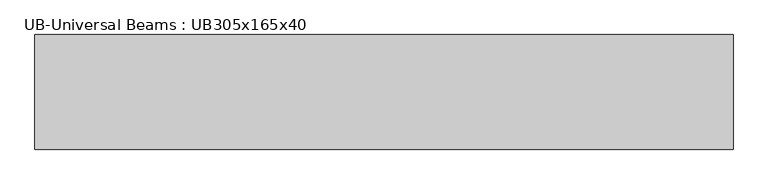
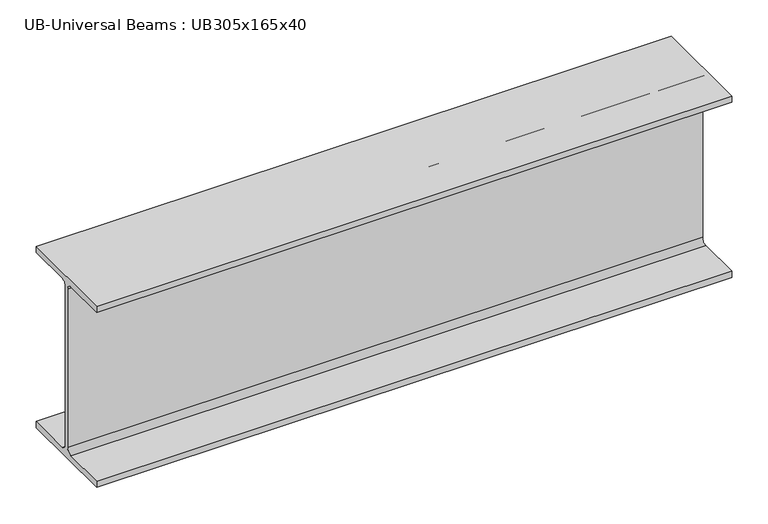
"""IFC4 building model written with IfcOpenShell, lengths in millimetres: beam geometry, UB-Universal Beams : UB305x165x40."""

from ifc_helpers import new_model, si_unit, point, frame, frame_2d, origin, place, context, project, spatial, polyline, circle_curve, trimmed, segment, composite_curve, outline, extrude, source, transform, mapped, element, save


def ub_universal_beams_ub305x165x40_23a6c5bf(model_context):
    return source(origin(), model_context, "Body", "SweptSolid", [
        extrude(outline(composite_curve([segment(polyline([(82.5, -141.5), (82.5, -151.7), (-82.5, -151.7), (-82.5, -141.5), (-11.9, -141.5)]), True, "CONTINUOUS"), segment(trimmed(circle_curve(frame_2d((-11.9, -132.6)), 8.9), [point((-11.9, -141.5))], [point((-3.0, -132.6))], True, "CARTESIAN"), True, "CONTINUOUS"), segment(polyline([(-3.0, -132.6), (-3.0, 132.6)]), True, "CONTINUOUS"), segment(trimmed(circle_curve(frame_2d((-11.9, 132.6)), 8.9), [point((-3.0, 132.6))], [point((-11.9, 141.5))], True, "CARTESIAN"), True, "CONTINUOUS"), segment(polyline([(-11.9, 141.5), (-82.5, 141.5), (-82.5, 151.7), (82.5, 151.7), (82.5, 141.5), (11.9, 141.5)]), True, "CONTINUOUS"), segment(trimmed(circle_curve(frame_2d((11.9, 132.6)), 8.9), [point((11.9, 141.5))], [point((3.0, 132.6))], True, "CARTESIAN"), True, "CONTINUOUS"), segment(polyline([(3.0, 132.6), (3.0, -132.6)]), True, "CONTINUOUS"), segment(trimmed(circle_curve(frame_2d((11.9, -132.6)), 8.9), [point((3.0, -132.6))], [point((11.9, -141.5))], True, "CARTESIAN"), True, "CONTINUOUS"), segment(polyline([(11.9, -141.5), (82.5, -141.5)]), True, "CONTINUOUS")], self_intersect=False)), frame((-672.8, 0.0, 0.0), z_axis=(1.0, 0.0, 0.0), x_axis=(0.0, 1.0, 0.0)), (0.0, 0.0, 1.0), 1004.9),
    ])


if __name__ == "__main__":
    model = new_model("IFC4")
    model_context = context("Model", 3, world=origin())
    ifc_project = project(units=[si_unit("LENGTHUNIT", "METRE", prefix="MILLI")], contexts=[model_context])
    site = spatial("IfcSite", under=ifc_project)
    building = spatial("IfcBuilding", under=site)
    placement = place(None, origin())
    ub_universal_beams_ub305x165x40_shape = ub_universal_beams_ub305x165x40_23a6c5bf(model_context)
    element("IfcBeam", 1, ObjectType="UB-Universal Beams : UB305x165x40", at=placement, inside=building, context=model_context, shape_type="MappedRepresentation", body=[
        mapped(ub_universal_beams_ub305x165x40_shape, transform((0.0, 0.0, 0.0), x_axis=(1.0, 0.0, 0.0), y_axis=(0.0, 1.0, 0.0), z_axis=(0.0, 0.0, 1.0))),
    ])
    save(model, "model.ifc")

# Revit data of these elements
# Type "UB-Universal Beams : UB305x165x40"
#   Section Name Key = "UB305X165X40"
#   Width = 16.5 cm
#   Web Thickness = 0.6 cm
#   Web Fillet = 0.89 cm
#   Warping Constant = 164000.0 cm⁶
#   Torsional Moment of Inertia = 14.70 cm⁴
#   Section Area = 51.3 cm²
#   Plastic Modulus weak axis = 142.0 cm³
#   Plastic Modulus strong axis = 623.0 cm³
#   Nominal Weight = 40.2999 kgf/m
#   Moment of Inertia weak axis = 764.00 cm⁴
#   Moment of Inertia strong axis = 8503.00 cm⁴
#   Height = 30.34 cm
#   Flange Thickness = 1.02 cm
#   Elastic Modulus weak axis = 92.6 cm³
#   Elastic Modulus strong axis = 560.0 cm³
#   Centroid Vertical = 15.17 cm
#   Centroid Horizontal = 8.25 cm
#   Bolt Spacing = 9.0 cm
#   Length [instance default] = 1500 mm
#   Structural Material [instance default] = Metal - Steel 43-275
#   Type Comments = ""
#   Assembly Code = ""
# Element 1 (IfcBeam, "UB-Universal Beams : UB305x165x40")
#   Materials on its faces: "Metal - Steel 43-275"
# Materials
#   "Metal - Steel 43-275": class "Metal", colour RGB 247 247 247, transparency 0, Cost = 0
